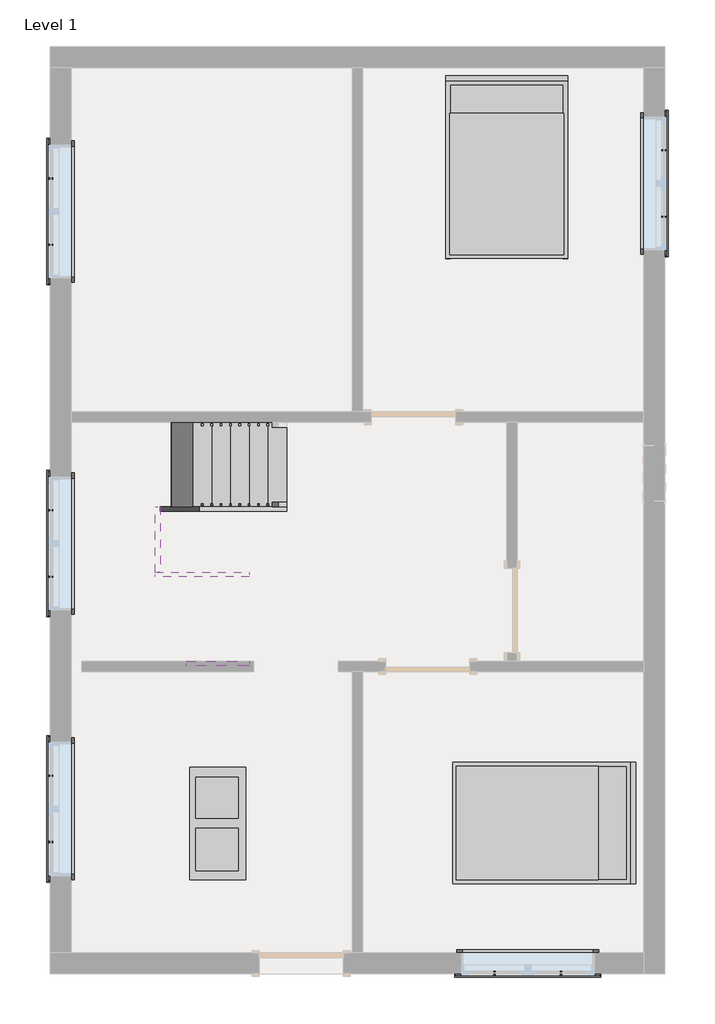
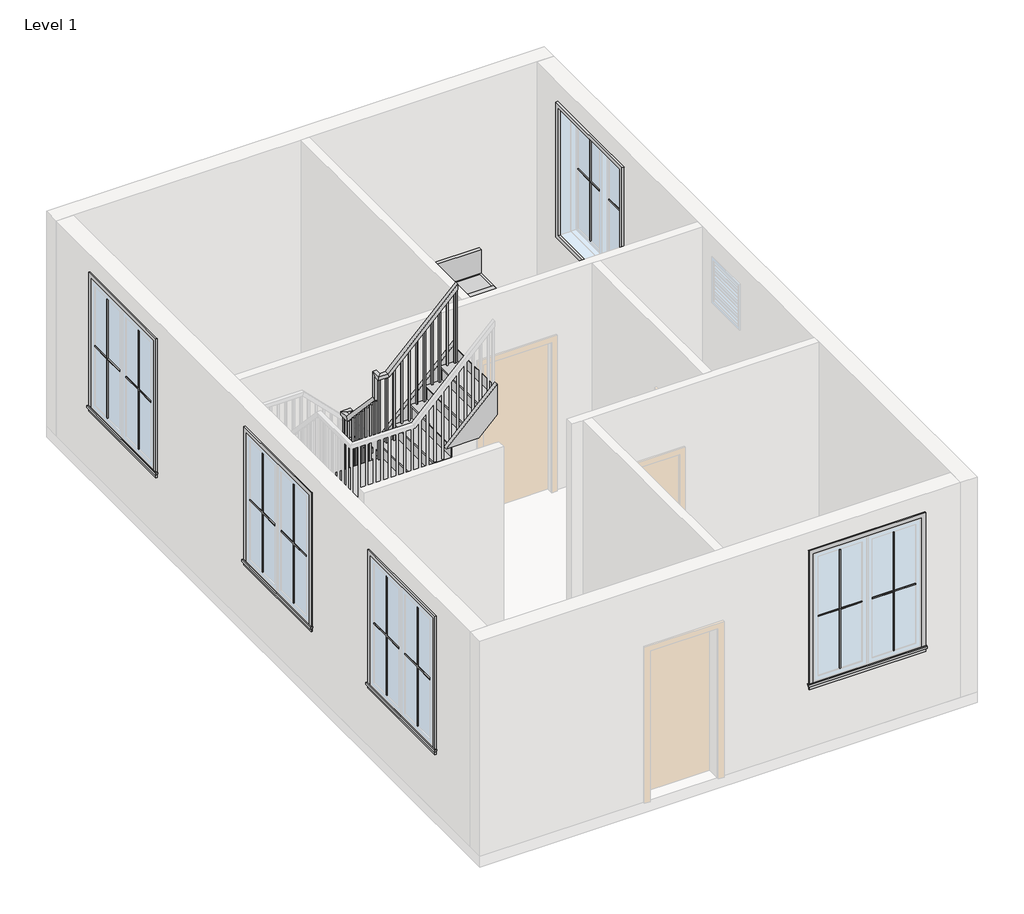
# One storey, part 2 of 2: 21 proxies, 5 members, 2 furniture elements, 1 railing, 1 stair flight.
"""IFC4 building model written with IfcOpenShell, lengths in millimetres."""

from ifc_helpers import new_model, si_unit, frame, origin, place, context, project, spatial, polyline, outline, extrude, faceted_brep, transform, mapped, element, save
from components import muntin_pattern_2x2_muntin_pattern_2x2_bff912c5, muntin_pattern_2x2_muntin_pattern_2x2_c2194282, trim_window_exterior_flat_with_sill_e04b3088, trim_window_interior_flat_picture_frame_2a7685fe, coffee_table_with_brass_mullions_11320_coffee_table_with_5962bef7, bed_17739_bed_17739_15c61121, stair_flight_8f890541

model = new_model("IFC4")

# Units and contexts
model_context = context("Model", 3, world=origin())
ifc_project = project(units=[si_unit("LENGTHUNIT", "METRE", prefix="MILLI")], contexts=[model_context])

# Site, building, storey
site = spatial("IfcSite", under=ifc_project)
building = spatial("IfcBuilding", under=site)
storey = spatial("IfcBuildingStorey", under=building, Name="Level 1", Elevation=0.0)

# Proxies
placement = place(None, origin())
muntin_pattern_2x2_muntin_pattern_2x2_shape = muntin_pattern_2x2_muntin_pattern_2x2_bff912c5(model_context)
element("IfcBuildingElementProxy", 1, Name="Muntin Pattern_2x2 : Muntin Pattern_2x2", ObjectType="Muntin Pattern_2x2 : Muntin Pattern_2x2", at=placement, inside=storey, context=model_context, shape_type="MappedRepresentation", body=[
    mapped(muntin_pattern_2x2_muntin_pattern_2x2_shape, transform((-626.5715247, -5050.1430046, 984.25), x_axis=(-1.0, 0.0, 0.0), y_axis=(0.0, -1.0, 0.0), z_axis=(0.0, 0.0, 1.0))),
])
element("IfcBuildingElementProxy", 2, Name="Muntin Pattern_2x2 : Muntin Pattern_2x2", ObjectType="Muntin Pattern_2x2 : Muntin Pattern_2x2", at=placement, inside=storey, context=model_context, shape_type="MappedRepresentation", body=[
    mapped(muntin_pattern_2x2_muntin_pattern_2x2_shape, transform((-6159.0090247, -3629.3305046, 984.25), x_axis=(0.0, 1.0, 0.0), y_axis=(-1.0, 0.0, 0.0), z_axis=(0.0, 0.0, 1.0))),
])
element("IfcBuildingElementProxy", 3, Name="Muntin Pattern_2x2 : Muntin Pattern_2x2", ObjectType="Muntin Pattern_2x2 : Muntin Pattern_2x2", at=placement, inside=storey, context=model_context, shape_type="MappedRepresentation", body=[
    mapped(muntin_pattern_2x2_muntin_pattern_2x2_shape, transform((489.4409753, 3873.1944954, 984.25), x_axis=(0.0, -1.0, 0.0), y_axis=(1.0, 0.0, 0.0), z_axis=(0.0, 0.0, 1.0))),
])
element("IfcBuildingElementProxy", 4, Name="Muntin Pattern_2x2 : Muntin Pattern_2x2", ObjectType="Muntin Pattern_2x2 : Muntin Pattern_2x2", at=placement, inside=storey, context=model_context, shape_type="MappedRepresentation", body=[
    mapped(muntin_pattern_2x2_muntin_pattern_2x2_shape, transform((-6159.0090247, 2847.6694954, 984.25), x_axis=(0.0, 1.0, 0.0), y_axis=(-1.0, 0.0, 0.0), z_axis=(0.0, 0.0, 1.0))),
])
element("IfcBuildingElementProxy", 5, Name="Muntin Pattern_2x2 : Muntin Pattern_2x2", ObjectType="Muntin Pattern_2x2 : Muntin Pattern_2x2", at=placement, inside=storey, context=model_context, shape_type="MappedRepresentation", body=[
    mapped(muntin_pattern_2x2_muntin_pattern_2x2_shape, transform((-6159.0090247, -752.7805046, 984.25), x_axis=(0.0, 1.0, 0.0), y_axis=(-1.0, 0.0, 0.0), z_axis=(0.0, 0.0, 1.0))),
])
muntin_pattern_2x2_muntin_pattern_2x2_2_shape = muntin_pattern_2x2_muntin_pattern_2x2_c2194282(model_context)
element("IfcBuildingElementProxy", 6, Name="Muntin Pattern_2x2 : Muntin Pattern_2x2", ObjectType="Muntin Pattern_2x2 : Muntin Pattern_2x2", at=placement, inside=storey, context=model_context, shape_type="MappedRepresentation", body=[
    mapped(muntin_pattern_2x2_muntin_pattern_2x2_2_shape, transform((-1347.2965247, -5050.1430046, 984.25), x_axis=(1.0, 0.0, 0.0), y_axis=(0.0, 1.0, 0.0), z_axis=(0.0, 0.0, 1.0))),
])
element("IfcBuildingElementProxy", 7, Name="Muntin Pattern_2x2 : Muntin Pattern_2x2", ObjectType="Muntin Pattern_2x2 : Muntin Pattern_2x2", at=placement, inside=storey, context=model_context, shape_type="MappedRepresentation", body=[
    mapped(muntin_pattern_2x2_muntin_pattern_2x2_2_shape, transform((-6159.0090247, -2908.6055046, 984.25), x_axis=(0.0, -1.0, 0.0), y_axis=(1.0, 0.0, 0.0), z_axis=(0.0, 0.0, 1.0))),
])
element("IfcBuildingElementProxy", 8, Name="Muntin Pattern_2x2 : Muntin Pattern_2x2", ObjectType="Muntin Pattern_2x2 : Muntin Pattern_2x2", at=placement, inside=storey, context=model_context, shape_type="MappedRepresentation", body=[
    mapped(muntin_pattern_2x2_muntin_pattern_2x2_2_shape, transform((489.4409753, 3152.4694954, 984.25), x_axis=(0.0, 1.0, 0.0), y_axis=(-1.0, 0.0, 0.0), z_axis=(0.0, 0.0, 1.0))),
])
element("IfcBuildingElementProxy", 9, Name="Muntin Pattern_2x2 : Muntin Pattern_2x2", ObjectType="Muntin Pattern_2x2 : Muntin Pattern_2x2", at=placement, inside=storey, context=model_context, shape_type="MappedRepresentation", body=[
    mapped(muntin_pattern_2x2_muntin_pattern_2x2_2_shape, transform((-6159.0090247, 3568.3944954, 984.25), x_axis=(0.0, -1.0, 0.0), y_axis=(1.0, 0.0, 0.0), z_axis=(0.0, 0.0, 1.0))),
])
element("IfcBuildingElementProxy", 10, Name="Muntin Pattern_2x2 : Muntin Pattern_2x2", ObjectType="Muntin Pattern_2x2 : Muntin Pattern_2x2", at=placement, inside=storey, context=model_context, shape_type="MappedRepresentation", body=[
    mapped(muntin_pattern_2x2_muntin_pattern_2x2_2_shape, transform((-6159.0090247, -32.0555046, 984.25), x_axis=(0.0, -1.0, 0.0), y_axis=(1.0, 0.0, 0.0), z_axis=(0.0, 0.0, 1.0))),
])
trim_window_exterior_flat_with_sill_shape = trim_window_exterior_flat_with_sill_e04b3088(model_context)
element("IfcBuildingElementProxy", 11, Name="Trim-Window-Exterior-Flat : with Sill", ObjectType="Trim-Window-Exterior-Flat : with Sill", at=placement, inside=storey, context=model_context, shape_type="MappedRepresentation", body=[
    mapped(trim_window_exterior_flat_with_sill_shape, transform((-986.9340247, -5059.6680046, 2743.2), x_axis=(1.0, 0.0, 0.0), y_axis=(0.0, 0.0, 1.0), z_axis=(0.0, -1.0, 0.0))),
])
element("IfcBuildingElementProxy", 12, Name="Trim-Window-Exterior-Flat : with Sill", ObjectType="Trim-Window-Exterior-Flat : with Sill", at=placement, inside=storey, context=model_context, shape_type="MappedRepresentation", body=[
    mapped(trim_window_exterior_flat_with_sill_shape, transform((-6168.5340247, -3268.9680046, 2743.2), x_axis=(0.0, -1.0, 0.0), y_axis=(0.0, 0.0, 1.0), z_axis=(-1.0, 0.0, 0.0))),
])
element("IfcBuildingElementProxy", 13, Name="Trim-Window-Exterior-Flat : with Sill", ObjectType="Trim-Window-Exterior-Flat : with Sill", at=placement, inside=storey, context=model_context, shape_type="MappedRepresentation", body=[
    mapped(trim_window_exterior_flat_with_sill_shape, transform((498.9659753, 3512.8319954, 2743.2), x_axis=(0.0, 1.0, 0.0), y_axis=(0.0, 0.0, 1.0), z_axis=(1.0, 0.0, 0.0))),
])
element("IfcBuildingElementProxy", 14, Name="Trim-Window-Exterior-Flat : with Sill", ObjectType="Trim-Window-Exterior-Flat : with Sill", at=placement, inside=storey, context=model_context, shape_type="MappedRepresentation", body=[
    mapped(trim_window_exterior_flat_with_sill_shape, transform((-6168.5340247, 3208.0319954, 2743.2), x_axis=(0.0, -1.0, 0.0), y_axis=(0.0, 0.0, 1.0), z_axis=(-1.0, 0.0, 0.0))),
])
element("IfcBuildingElementProxy", 15, Name="Trim-Window-Exterior-Flat : with Sill", ObjectType="Trim-Window-Exterior-Flat : with Sill", at=placement, inside=storey, context=model_context, shape_type="MappedRepresentation", body=[
    mapped(trim_window_exterior_flat_with_sill_shape, transform((-6168.5340247, -392.4180046, 2743.2), x_axis=(0.0, -1.0, 0.0), y_axis=(0.0, 0.0, 1.0), z_axis=(-1.0, 0.0, 0.0))),
])
trim_window_interior_flat_picture_frame_shape = trim_window_interior_flat_picture_frame_2a7685fe(model_context)
element("IfcBuildingElementProxy", 16, Name="Trim-Window-Interior-Flat : Picture Frame", ObjectType="Trim-Window-Interior-Flat : Picture Frame", at=placement, inside=storey, context=model_context, shape_type="MappedRepresentation", body=[
    mapped(trim_window_interior_flat_picture_frame_shape, transform((-986.9340247, -4831.0680046, 2743.2), x_axis=(-1.0, 0.0, 0.0), y_axis=(0.0, 0.0, 1.0), z_axis=(0.0, 1.0, 0.0))),
])
element("IfcBuildingElementProxy", 17, Name="Trim-Window-Interior-Flat : Picture Frame", ObjectType="Trim-Window-Interior-Flat : Picture Frame", at=placement, inside=storey, context=model_context, shape_type="MappedRepresentation", body=[
    mapped(trim_window_interior_flat_picture_frame_shape, transform((-5939.9340247, -3268.9680046, 2743.2), x_axis=(0.0, 1.0, 0.0), y_axis=(0.0, 0.0, 1.0), z_axis=(1.0, 0.0, 0.0))),
])
element("IfcBuildingElementProxy", 18, Name="Trim-Window-Interior-Flat : Picture Frame", ObjectType="Trim-Window-Interior-Flat : Picture Frame", at=placement, inside=storey, context=model_context, shape_type="MappedRepresentation", body=[
    mapped(trim_window_interior_flat_picture_frame_shape, transform((270.3659753, 3512.8319954, 2743.2), x_axis=(0.0, -1.0, 0.0), y_axis=(0.0, 0.0, 1.0), z_axis=(-1.0, 0.0, 0.0))),
])
element("IfcBuildingElementProxy", 19, Name="Trim-Window-Interior-Flat : Picture Frame", ObjectType="Trim-Window-Interior-Flat : Picture Frame", at=placement, inside=storey, context=model_context, shape_type="MappedRepresentation", body=[
    mapped(trim_window_interior_flat_picture_frame_shape, transform((-5939.9340247, 3208.0319954, 2743.2), x_axis=(0.0, 1.0, 0.0), y_axis=(0.0, 0.0, 1.0), z_axis=(1.0, 0.0, 0.0))),
])
element("IfcBuildingElementProxy", 20, Name="Trim-Window-Interior-Flat : Picture Frame", ObjectType="Trim-Window-Interior-Flat : Picture Frame", at=placement, inside=storey, context=model_context, shape_type="MappedRepresentation", body=[
    mapped(trim_window_interior_flat_picture_frame_shape, transform((-5939.9340247, -392.4180046, 2743.2), x_axis=(0.0, 1.0, 0.0), y_axis=(0.0, 0.0, 1.0), z_axis=(1.0, 0.0, 0.0))),
])
coffee_table_with_brass_mullions_11320_coffee_table_with_shape = coffee_table_with_brass_mullions_11320_coffee_table_with_5962bef7(model_context)
element("IfcBuildingElementProxy", 21, Name="coffee_table_with_brass_mullions_11320 : coffee_table_with_brass_mullions_11320", ObjectType="coffee_table_with_brass_mullions_11320 : coffee_table_with_brass_mullions_11320", at=placement, inside=storey, context=model_context, shape_type="MappedRepresentation", body=[
    mapped(coffee_table_with_brass_mullions_11320_coffee_table_with_shape, transform((-3920.6340247, -2792.7180046, 0.0), x_axis=(0.0, 1.0, 0.0), y_axis=(-1.0, 0.0, 0.0), z_axis=(0.0, 0.0, 1.0))),
])

# Furniture
bed_17739_bed_17739_shape = bed_17739_bed_17739_15c61121(model_context)
element("IfcFurniture", 22, ObjectType="Bed_17739 : Bed_17739", at=placement, inside=storey, context=model_context, shape_type="MappedRepresentation", body=[
    mapped(bed_17739_bed_17739_shape, transform((-1215.5340247, 3665.2319954, 0.0), x_axis=(1.0, 0.0, 0.0), y_axis=(0.0, 1.0, 0.0), z_axis=(0.0, 0.0, 1.0))),
])
element("IfcFurniture", 23, ObjectType="Bed_17739 : Bed_17739", at=placement, inside=storey, context=model_context, shape_type="MappedRepresentation", body=[
    mapped(bed_17739_bed_17739_shape, transform((-834.5340247, -3421.3680046, 0.0), x_axis=(0.0, -1.0, 0.0), y_axis=(1.0, 0.0, 0.0), z_axis=(0.0, 0.0, 1.0))),
])

# Members
element("IfcMember", 24, ObjectType="Stringer - 2\" Width", at=placement, inside=storey, context=model_context, shape_type="SweptSolid", body=[
    extrude(outline(polyline([(0.0, -3603.1340247), (258.6997326, -3603.1340247), (1630.2997326, -4974.7340247), (1199.2474388, -4974.7340247), (0.0, -3775.4865859), (0.0, -3603.1340247)])), frame((0.0, -43.1680046, 0.0), z_axis=(0.0, 1.0, 0.0), x_axis=(0.0, 0.0, 1.0)), (0.0, 0.0, 1.0), 50.8),
])
element("IfcMember", 25, ObjectType="Stringer - 2\" Width", at=placement, inside=storey, context=model_context, shape_type="SweptSolid", body=[
    extrude(outline(polyline([(7.6319954, 1893.7414769), (7.6319954, 1448.089085), (-703.5680046, 2206.7024184), (-703.5680046, 2652.3548102), (7.6319954, 1893.7414769)])), frame((-5025.5340247, 0.0, 0.0), z_axis=(1.0, 0.0, 0.0), x_axis=(0.0, 1.0, 0.0)), (0.0, 0.0, 1.0), 50.8),
])
element("IfcMember", 26, ObjectType="Stringer - 2\" Width", at=placement, inside=storey, context=model_context, shape_type="SweptSolid", body=[
    extrude(outline(polyline([(2900.2997326, -5025.5340247), (2469.2474388, -5025.5340247), (3485.2474388, -4009.5340247), (3916.2997326, -4009.5340247), (2900.2997326, -5025.5340247)])), frame((0.0, -754.3680046, 0.0), z_axis=(0.0, 1.0, 0.0), x_axis=(0.0, 0.0, 1.0)), (0.0, 0.0, 1.0), 50.8),
])
element("IfcMember", 27, ObjectType="Stringer - 2\" Width", at=placement, inside=storey, context=model_context, shape_type="SweptSolid", body=[
    extrude(outline(polyline([(0.0, -3603.1340247), (258.6997326, -3603.1340247), (918.3814769, -4262.815769), (918.3814769, -4693.8680628), (0.0, -3775.4865859), (0.0, -3603.1340247)])), frame((0.0, 922.0319954, 0.0), z_axis=(0.0, 1.0, 0.0), x_axis=(0.0, 0.0, 1.0)), (0.0, 0.0, 1.0), 50.8),
])
element("IfcMember", 28, ObjectType="Stringer - 2\" Width", at=placement, inside=storey, context=model_context, shape_type="SweptSolid", body=[
    extrude(outline(polyline([(3236.249085, -4258.5323784), (3485.2474388, -4009.5340247), (3916.2997326, -4009.5340247), (3236.249085, -4689.5846723), (3236.249085, -4258.5323784)])), frame((0.0, -1719.5680046, 0.0), z_axis=(0.0, 1.0, 0.0), x_axis=(0.0, 0.0, 1.0)), (0.0, 0.0, 1.0), 50.8),
])

# Railing
element("IfcRailing", 29, ObjectType="Handrail - Rectangular", at=placement, inside=storey, context=model_context, shape_type="SolidModel", body=[
    faceted_brep([(-3603.1340247, 7.6319954, 1117.6), (-3603.1340247, 7.6319954, 1045.757951), (-3603.1340247, 58.4319954, 1045.757951), (-3603.1340247, 58.4319954, 1117.6), (-4949.3340247, 7.6319954, 2463.8), (-5000.1340247, 7.6319954, 2442.757951), (-5000.1340247, 58.4319954, 2442.757951), (-4949.3340247, 58.4319954, 2463.8), (-4949.3340247, 7.6319954, 2824.48), (-5000.1340247, 7.6319954, 2773.68), (-5000.1340247, 58.4319954, 2773.68), (-4949.3340247, 58.4319954, 2824.48), (-5025.5340247, 7.6319954, 2824.48), (-5025.5340247, 7.6319954, 2773.68), (-5076.3340247, 58.4319954, 2773.68), (-5076.3340247, 58.4319954, 2824.48), (-5025.5340247, -68.5680046, 2824.48), (-5025.5340247, -90.5761909, 2773.68), (-5076.3340247, -90.5761909, 2773.68), (-5076.3340247, -68.5680046, 2824.48), (-5025.5340247, -678.1680046, 3474.72), (-5025.5340247, -728.9680046, 3454.631268), (-5076.3340247, -728.9680046, 3454.631268), (-5076.3340247, -678.1680046, 3474.72), (-5025.5340247, -678.1680046, 3835.4), (-5025.5340247, -728.9680046, 3784.6), (-5076.3340247, -728.9680046, 3784.6), (-5076.3340247, -678.1680046, 3835.4), (-5025.5340247, -754.3680046, 3835.4), (-5025.5340247, -754.3680046, 3784.6), (-5076.3340247, -805.1680046, 3784.6), (-5076.3340247, -805.1680046, 3835.4), (-4949.3340247, -754.3680046, 3835.4), (-4928.2919757, -754.3680046, 3784.6), (-4928.2919757, -805.1680046, 3784.6), (-4949.3340247, -805.1680046, 3835.4), (-4009.5340247, -754.3680046, 4775.2), (-4009.5340247, -805.1680046, 4775.2), (-4009.5340247, -805.1680046, 4703.357951), (-4009.5340247, -754.3680046, 4703.357951)], [[[0, 1, 2, 3]], [[1, 0, 4, 5]], [[2, 1, 5, 6]], [[3, 2, 6, 7]], [[0, 3, 7, 4]], [[5, 4, 8, 9]], [[6, 5, 9, 10]], [[7, 6, 10, 11]], [[4, 7, 11, 8]], [[9, 8, 12, 13]], [[10, 9, 13, 14]], [[11, 10, 14, 15]], [[8, 11, 15, 12]], [[13, 12, 16, 17]], [[14, 13, 17, 18]], [[15, 14, 18, 19]], [[12, 15, 19, 16]], [[17, 16, 20, 21]], [[18, 17, 21, 22]], [[19, 18, 22, 23]], [[16, 19, 23, 20]], [[21, 20, 24, 25]], [[22, 21, 25, 26]], [[23, 22, 26, 27]], [[20, 23, 27, 24]], [[25, 24, 28, 29]], [[26, 25, 29, 30]], [[27, 26, 30, 31]], [[24, 27, 31, 28]], [[29, 28, 32, 33]], [[30, 29, 33, 34]], [[31, 30, 34, 35]], [[28, 31, 35, 32]], [[36, 37, 38, 39]], [[33, 32, 36, 39]], [[34, 33, 39, 38]], [[35, 34, 38, 37]], [[32, 35, 37, 36]]]),
    extrude(outline(polyline([(4668.432951, -4044.4590247), (3657.6, -4044.4590247), (3657.6, -4025.4090247), (4687.482951, -4025.4090247), (4668.432951, -4044.4590247)])), frame((0.0, -789.2930046, 0.0), z_axis=(0.0, 1.0, 0.0), x_axis=(0.0, 0.0, 1.0)), (0.0, 0.0, 1.0), 19.05),
    extrude(outline(polyline([(4566.832951, -4146.0590247), (3657.6, -4146.0590247), (3657.6, -4127.0090247), (4585.882951, -4127.0090247), (4566.832951, -4146.0590247)])), frame((0.0, -789.2930046, 0.0), z_axis=(0.0, 1.0, 0.0), x_axis=(0.0, 0.0, 1.0)), (0.0, 0.0, 1.0), 19.05),
    extrude(outline(polyline([(4465.232951, -4247.6590247), (3454.4, -4247.6590247), (3454.4, -4228.6090247), (4484.282951, -4228.6090247), (4465.232951, -4247.6590247)])), frame((0.0, -789.2930046, 0.0), z_axis=(0.0, 1.0, 0.0), x_axis=(0.0, 0.0, 1.0)), (0.0, 0.0, 1.0), 19.05),
    extrude(outline(polyline([(4363.632951, -4349.2590247), (3454.4, -4349.2590247), (3454.4, -4330.2090247), (4382.682951, -4330.2090247), (4363.632951, -4349.2590247)])), frame((0.0, -789.2930046, 0.0), z_axis=(0.0, 1.0, 0.0), x_axis=(0.0, 0.0, 1.0)), (0.0, 0.0, 1.0), 19.05),
    extrude(outline(polyline([(4262.032951, -4450.8590247), (3251.2, -4450.8590247), (3251.2, -4431.8090247), (4281.082951, -4431.8090247), (4262.032951, -4450.8590247)])), frame((0.0, -789.2930046, 0.0), z_axis=(0.0, 1.0, 0.0), x_axis=(0.0, 0.0, 1.0)), (0.0, 0.0, 1.0), 19.05),
    extrude(outline(polyline([(4160.432951, -4552.4590247), (3251.2, -4552.4590247), (3251.2, -4533.4090247), (4179.482951, -4533.4090247), (4160.432951, -4552.4590247)])), frame((0.0, -789.2930046, 0.0), z_axis=(0.0, 1.0, 0.0), x_axis=(0.0, 0.0, 1.0)), (0.0, 0.0, 1.0), 19.05),
    extrude(outline(polyline([(4058.832951, -4654.0590247), (3048.0, -4654.0590247), (3048.0, -4635.0090247), (4077.882951, -4635.0090247), (4058.832951, -4654.0590247)])), frame((0.0, -789.2930046, 0.0), z_axis=(0.0, 1.0, 0.0), x_axis=(0.0, 0.0, 1.0)), (0.0, 0.0, 1.0), 19.05),
    extrude(outline(polyline([(3957.232951, -4755.6590247), (3048.0, -4755.6590247), (3048.0, -4736.6090247), (3976.282951, -4736.6090247), (3957.232951, -4755.6590247)])), frame((0.0, -789.2930046, 0.0), z_axis=(0.0, 1.0, 0.0), x_axis=(0.0, 0.0, 1.0)), (0.0, 0.0, 1.0), 19.05),
    extrude(outline(polyline([(3855.632951, -4857.2590247), (2844.8, -4857.2590247), (2844.8, -4838.2090247), (3874.682951, -4838.2090247), (3855.632951, -4857.2590247)])), frame((0.0, -789.2930046, 0.0), z_axis=(0.0, 1.0, 0.0), x_axis=(0.0, 0.0, 1.0)), (0.0, 0.0, 1.0), 19.05),
    extrude(outline(polyline([(3754.032951, -4958.8590247), (2844.8, -4958.8590247), (2844.8, -4939.8090247), (3773.082951, -4939.8090247), (3754.032951, -4958.8590247)])), frame((0.0, -789.2930046, 0.0), z_axis=(0.0, 1.0, 0.0), x_axis=(0.0, 0.0, 1.0)), (0.0, 0.0, 1.0), 19.05),
    extrude(outline(polyline([(-668.6430046, 3390.2846014), (-668.6430046, 2438.4), (-687.6930046, 2438.4), (-687.6930046, 3410.6046014), (-668.6430046, 3390.2846014)])), frame((-5060.4590247, 0.0, 0.0), z_axis=(1.0, 0.0, 0.0), x_axis=(0.0, 1.0, 0.0)), (0.0, 0.0, 1.0), 19.05),
    extrude(outline(polyline([(-567.0430046, 3281.911268), (-567.0430046, 2438.4), (-586.0930046, 2438.4), (-586.0930046, 3302.231268), (-567.0430046, 3281.911268)])), frame((-5060.4590247, 0.0, 0.0), z_axis=(1.0, 0.0, 0.0), x_axis=(0.0, 1.0, 0.0)), (0.0, 0.0, 1.0), 19.05),
    extrude(outline(polyline([(-465.4430046, 3173.5379347), (-465.4430046, 2235.2), (-484.4930046, 2235.2), (-484.4930046, 3193.8579347), (-465.4430046, 3173.5379347)])), frame((-5060.4590247, 0.0, 0.0), z_axis=(1.0, 0.0, 0.0), x_axis=(0.0, 1.0, 0.0)), (0.0, 0.0, 1.0), 19.05),
    extrude(outline(polyline([(-363.8430046, 3065.1646014), (-363.8430046, 2235.2), (-382.8930046, 2235.2), (-382.8930046, 3085.4846014), (-363.8430046, 3065.1646014)])), frame((-5060.4590247, 0.0, 0.0), z_axis=(1.0, 0.0, 0.0), x_axis=(0.0, 1.0, 0.0)), (0.0, 0.0, 1.0), 19.05),
    extrude(outline(polyline([(-262.2430046, 2956.791268), (-262.2430046, 2032.0), (-281.2930046, 2032.0), (-281.2930046, 2977.111268), (-262.2430046, 2956.791268)])), frame((-5060.4590247, 0.0, 0.0), z_axis=(1.0, 0.0, 0.0), x_axis=(0.0, 1.0, 0.0)), (0.0, 0.0, 1.0), 19.05),
    extrude(outline(polyline([(-160.6430046, 2848.4179347), (-160.6430046, 2032.0), (-179.6930046, 2032.0), (-179.6930046, 2868.7379347), (-160.6430046, 2848.4179347)])), frame((-5060.4590247, 0.0, 0.0), z_axis=(1.0, 0.0, 0.0), x_axis=(0.0, 1.0, 0.0)), (0.0, 0.0, 1.0), 19.05),
    extrude(outline(polyline([(-59.0430046, 2740.0446014), (-59.0430046, 1828.8), (-78.0930046, 1828.8), (-78.0930046, 2760.3646014), (-59.0430046, 2740.0446014)])), frame((-5060.4590247, 0.0, 0.0), z_axis=(1.0, 0.0, 0.0), x_axis=(0.0, 1.0, 0.0)), (0.0, 0.0, 1.0), 19.05),
    extrude(outline(polyline([(-5016.0090247, 23.5069954), (-5035.0590247, 23.5069954), (-5035.0590247, 42.5569954), (-5016.0090247, 42.5569954), (-5016.0090247, 23.5069954)])), frame((0.0, 0.0, 1625.6), z_axis=(0.0, 0.0, 1.0), x_axis=(1.0, 0.0, 0.0)), (0.0, 0.0, 1.0), 1148.08),
    extrude(outline(polyline([(2376.082951, -4933.4590247), (1422.4, -4933.4590247), (1422.4, -4914.4090247), (2357.032951, -4914.4090247), (2376.082951, -4933.4590247)])), frame((0.0, 23.5069954, 0.0), z_axis=(0.0, 1.0, 0.0), x_axis=(0.0, 0.0, 1.0)), (0.0, 0.0, 1.0), 19.05),
    extrude(outline(polyline([(2274.482951, -4831.8590247), (1422.4, -4831.8590247), (1422.4, -4812.8090247), (2255.432951, -4812.8090247), (2274.482951, -4831.8590247)])), frame((0.0, 23.5069954, 0.0), z_axis=(0.0, 1.0, 0.0), x_axis=(0.0, 0.0, 1.0)), (0.0, 0.0, 1.0), 19.05),
    extrude(outline(polyline([(2172.882951, -4730.2590247), (1219.2, -4730.2590247), (1219.2, -4711.2090247), (2153.832951, -4711.2090247), (2172.882951, -4730.2590247)])), frame((0.0, 23.5069954, 0.0), z_axis=(0.0, 1.0, 0.0), x_axis=(0.0, 0.0, 1.0)), (0.0, 0.0, 1.0), 19.05),
    extrude(outline(polyline([(2071.282951, -4628.6590247), (1219.2, -4628.6590247), (1219.2, -4609.6090247), (2052.232951, -4609.6090247), (2071.282951, -4628.6590247)])), frame((0.0, 23.5069954, 0.0), z_axis=(0.0, 1.0, 0.0), x_axis=(0.0, 0.0, 1.0)), (0.0, 0.0, 1.0), 19.05),
    extrude(outline(polyline([(1969.682951, -4527.0590247), (1016.0, -4527.0590247), (1016.0, -4508.0090247), (1950.632951, -4508.0090247), (1969.682951, -4527.0590247)])), frame((0.0, 23.5069954, 0.0), z_axis=(0.0, 1.0, 0.0), x_axis=(0.0, 0.0, 1.0)), (0.0, 0.0, 1.0), 19.05),
    extrude(outline(polyline([(1868.082951, -4425.4590247), (1016.0, -4425.4590247), (1016.0, -4406.4090247), (1849.032951, -4406.4090247), (1868.082951, -4425.4590247)])), frame((0.0, 23.5069954, 0.0), z_axis=(0.0, 1.0, 0.0), x_axis=(0.0, 0.0, 1.0)), (0.0, 0.0, 1.0), 19.05),
    extrude(outline(polyline([(1766.482951, -4323.8590247), (812.8, -4323.8590247), (812.8, -4304.8090247), (1747.432951, -4304.8090247), (1766.482951, -4323.8590247)])), frame((0.0, 23.5069954, 0.0), z_axis=(0.0, 1.0, 0.0), x_axis=(0.0, 0.0, 1.0)), (0.0, 0.0, 1.0), 19.05),
    extrude(outline(polyline([(1664.882951, -4222.2590247), (812.8, -4222.2590247), (812.8, -4203.2090247), (1645.832951, -4203.2090247), (1664.882951, -4222.2590247)])), frame((0.0, 23.5069954, 0.0), z_axis=(0.0, 1.0, 0.0), x_axis=(0.0, 0.0, 1.0)), (0.0, 0.0, 1.0), 19.05),
    extrude(outline(polyline([(1563.282951, -4120.6590247), (609.6, -4120.6590247), (609.6, -4101.6090247), (1544.232951, -4101.6090247), (1563.282951, -4120.6590247)])), frame((0.0, 23.5069954, 0.0), z_axis=(0.0, 1.0, 0.0), x_axis=(0.0, 0.0, 1.0)), (0.0, 0.0, 1.0), 19.05),
    extrude(outline(polyline([(1461.682951, -4019.0590247), (609.6, -4019.0590247), (609.6, -4000.0090247), (1442.632951, -4000.0090247), (1461.682951, -4019.0590247)])), frame((0.0, 23.5069954, 0.0), z_axis=(0.0, 1.0, 0.0), x_axis=(0.0, 0.0, 1.0)), (0.0, 0.0, 1.0), 19.05),
    extrude(outline(polyline([(1360.082951, -3917.4590247), (406.4, -3917.4590247), (406.4, -3898.4090247), (1341.032951, -3898.4090247), (1360.082951, -3917.4590247)])), frame((0.0, 23.5069954, 0.0), z_axis=(0.0, 1.0, 0.0), x_axis=(0.0, 0.0, 1.0)), (0.0, 0.0, 1.0), 19.05),
    extrude(outline(polyline([(1258.482951, -3815.8590247), (406.4, -3815.8590247), (406.4, -3796.8090247), (1239.432951, -3796.8090247), (1258.482951, -3815.8590247)])), frame((0.0, 23.5069954, 0.0), z_axis=(0.0, 1.0, 0.0), x_axis=(0.0, 0.0, 1.0)), (0.0, 0.0, 1.0), 19.05),
    extrude(outline(polyline([(1156.882951, -3714.2590247), (203.2, -3714.2590247), (203.2, -3695.2090247), (1137.832951, -3695.2090247), (1156.882951, -3714.2590247)])), frame((0.0, 23.5069954, 0.0), z_axis=(0.0, 1.0, 0.0), x_axis=(0.0, 0.0, 1.0)), (0.0, 0.0, 1.0), 19.05),
    extrude(outline(polyline([(-5041.4090247, -770.2430046), (-5041.4090247, -789.2930046), (-5060.4590247, -789.2930046), (-5060.4590247, -770.2430046), (-5041.4090247, -770.2430046)])), frame((0.0, 0.0, 2641.6), z_axis=(0.0, 0.0, 1.0), x_axis=(1.0, 0.0, 0.0)), (0.0, 0.0, 1.0), 1143.0),
    extrude(outline(polyline([(-5041.4090247, 23.5069954), (-5060.4590247, 23.5069954), (-5060.4590247, 42.5569954), (-5041.4090247, 42.5569954), (-5041.4090247, 23.5069954)])), frame((0.0, 0.0, 1625.6), z_axis=(0.0, 0.0, 1.0), x_axis=(1.0, 0.0, 0.0)), (0.0, 0.0, 1.0), 1148.08),
    extrude(outline(polyline([(4684.307951, -4028.5840247), (3657.6, -4028.5840247), (3657.6, -4009.5340247), (4703.357951, -4009.5340247), (4684.307951, -4028.5840247)])), frame((0.0, -789.2930046, 0.0), z_axis=(0.0, 1.0, 0.0), x_axis=(0.0, 0.0, 1.0)), (0.0, 0.0, 1.0), 19.05),
    extrude(outline(polyline([(1064.807951, -3622.1840247), (203.2, -3622.1840247), (203.2, -3603.1340247), (1045.757951, -3603.1340247), (1064.807951, -3622.1840247)])), frame((0.0, 23.5069954, 0.0), z_axis=(0.0, 1.0, 0.0), x_axis=(0.0, 0.0, 1.0)), (0.0, 0.0, 1.0), 19.05),
])

# Stair flight
stair_flight_shape = stair_flight_8f890541(model_context)
element("IfcStairFlight", 30, ObjectType="2\" Tread 1\" Nosing 1/4\" Riser", at=placement, inside=storey, context=model_context, shape_type="MappedRepresentation", body=[
    mapped(stair_flight_shape, transform((0.0, 0.0, 0.0), x_axis=(1.0, 0.0, 0.0), y_axis=(0.0, 1.0, 0.0), z_axis=(0.0, 0.0, 1.0))),
])

save(model, "model.ifc")

# Revit data of these elements
# Type "Muntin Pattern_2x2 : Muntin Pattern_2x2"
#   Width [instance default] = 4' - 0"
#   Thickness = 0' - 0 1/2"
#   Height [instance default] = 4' - 0"
#   Distance = 0' - 0 3/4"
#   Interior Material [instance default] = none
#   Exterior Material [instance default] = none
#   Default Elevation = 0
# Type "Trim-Window-Exterior-Flat : with Sill"
#   Trim Width = 0' - 2 1/4"
#   Trim Thickness_Picture Frame = 0' - 1 1/4"
#   Trim Thickness_with Sill = 0' - 0 3/4"
#   Sill Thickness = 0' - 1 1/4"
#   Opening Width [instance default] = 2' - 0"
#   Opening Height [instance default] = 3' - 0"
#   Default Elevation = 4' - 0"
#   Sill = yes
#   Picture Frame = no
#   Trim Material [instance default] = none
# Type "Trim-Window-Interior-Flat : Picture Frame"
#   Trim Thickness_Picture Frame = 0' - 1 1/4"
#   Trim Width = 0' - 2 1/4"
#   Trim Thickness_with Sill = 0' - 0 3/4"
#   Sill Thickness = 0' - 1 1/4"
#   Opening Width [instance default] = 2' - 0"
#   Opening Height [instance default] = 3' - 0"
#   Default Elevation = 4' - 0"
#   Sill = no
#   Picture Frame = yes
#   Trim Material [instance default] = none
# Type "coffee_table_with_brass_mullions_11320 : coffee_table_with_brass_mullions_11320"
#   Default Elevation = 0
# Type "Bed_17739 : Bed_17739"
#   Default Elevation = 0
# Type "Handrail - Rectangular"
#   Assembly Code = "C2010400"
#   built-in parameter 1008612 = 0.0416667 (stored number, unit not read)
#   built-in parameter 1008611 = 0.0416667 (stored number, unit not read)
#   built-in parameter 1008609 = 0.333333 (stored number, unit not read)
#   built-in parameter 1008604 = 0.166667 (stored number, unit not read)
#   built-in parameter 1008603 = 0.166667 (stored number, unit not read)
#   Railing Height = 3' - 0"
#   built-in parameter 1008630 = 2
#   built-in parameter 1008610 = 2
#   built-in parameter 1008618 = Baluster - Square : 3/4"
# Elements 1, 2, 3, 4, 5, 6, 7, 8, 9, 10 (IfcBuildingElementProxy, "Muntin Pattern_2x2 : Muntin Pattern_2x2")
#   Width = 1' - 11 1/8"
#   Height = 5' - 6 1/2"
#   Interior Material = Wood - Stained
#   Exterior Material = Clad - White
#   Phase Created = New Construction
#   Materials on its faces: "Clad - White", "Wood - Stained"
# Elements 11, 12, 13, 14, 15 (IfcBuildingElementProxy, "Trim-Window-Exterior-Flat : with Sill")
#   Opening Width = 4' - 9"
#   Opening Height = 6' - 0"
#   Trim Material = Clad - White
#   Phase Created = New Construction
#   Materials on its faces: "Clad - White"
# Elements 16, 17, 18, 19, 20 (IfcBuildingElementProxy, "Trim-Window-Interior-Flat : Picture Frame")
#   Opening Width = 4' - 9"
#   Opening Height = 6' - 0"
#   Trim Material = Wood - Stained
#   Phase Created = New Construction
#   Materials on its faces: "Wood - Stained"
# Element 21 (IfcBuildingElementProxy, "coffee_table_with_brass_mullions_11320 : coffee_table_with_brass_mullions_11320")
#   Phase Created = New Construction
#   Materials on its faces: "Default Wall", "TABLE", "Glass", "Default"
# Elements 22, 23 (IfcFurniture, "Bed_17739 : Bed_17739")
#   Phase Created = New Construction
#   Materials on its faces: "legs", "sheets", "bed frame", "Blanket"
# Elements 24, 25, 26, 27, 28 (IfcMember, "Stringer - 2\" Width")
#   Phase Created = New Construction
# Element 29 (IfcRailing, "Handrail - Rectangular")
#   Phase Created = New Construction
#   Materials on its faces: "Oak Flooring"
# Element 30 (IfcStairFlight, "2\" Tread 1\" Nosing 1/4\" Riser")
#   Phase Created = New Construction
# Materials
#   "Clad - White": class "Wood", colour RGB 242 242 238, transparency 0, Cost = 0
#   "Wood - Stained": class "Wood", colour RGB 224 178 126, transparency 0, Cost = 0
#   "Default Wall": colour RGB 128 128 128, transparency 0, Cost = 0
#   "TABLE": class "Generic", colour RGB 120 120 120, transparency 0, Cost = 0
#   "Glass": class "Glass", colour RGB 0 128 192, transparency 0.75, Description = "Soda Lime Glass", Cost = 0
#   "Default": colour RGB 127 127 127, transparency 0, Cost = 0
#   "legs": colour RGB 90 73 37, transparency 0, Cost = 0
#   "sheets": colour RGB 200 195 176, transparency 0, Cost = 0
#   "bed frame": colour RGB 90 73 37, transparency 0, Cost = 0
#   "Blanket": class "System", colour RGB 59 0 1, transparency 0, Cost = 0
#   "Oak Flooring": class "Wood", colour RGB 216 169 114, transparency 0, Description = "Quercus Rubra", Cost = 0
